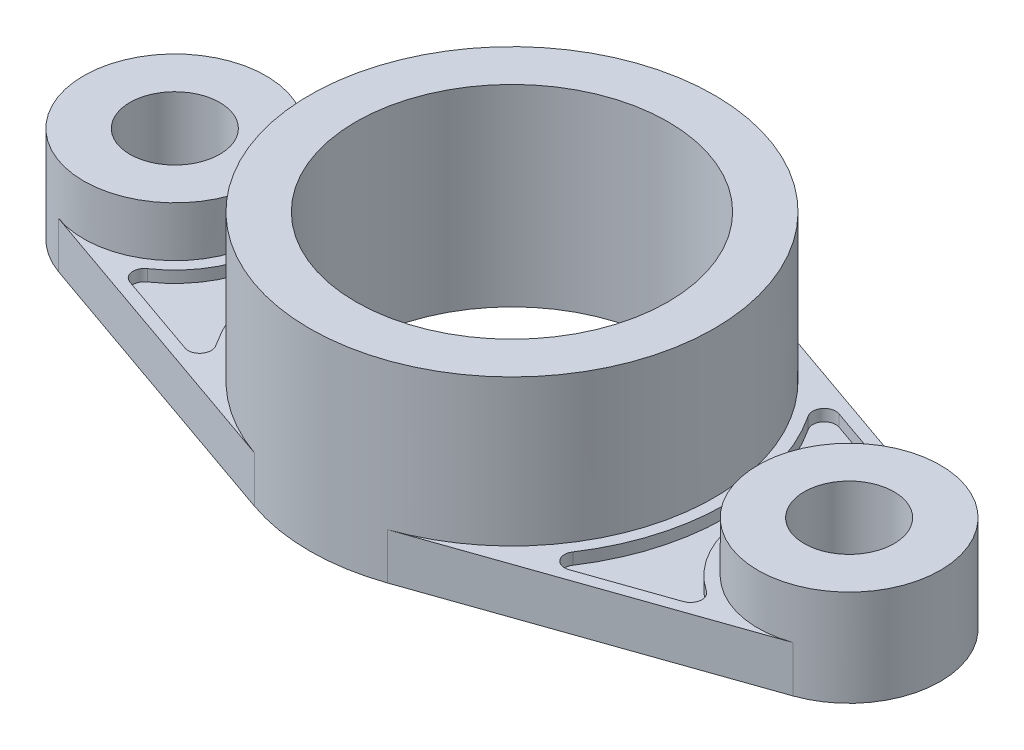
ISO-10303-21;
HEADER;
FILE_DESCRIPTION(('STEP AP214'),'2;1');
FILE_NAME('part.step','',(''),(''),'','','');
FILE_SCHEMA(('AUTOMOTIVE_DESIGN { 1 0 10303 214 1 1 1 1 }'));
ENDSEC;
DATA;
#1=APPLICATION_CONTEXT('core data for automotive mechanical design processes');
#2=APPLICATION_PROTOCOL_DEFINITION('international standard','automotive_design',2000,#1);
#3=PRODUCT_CONTEXT('',#1,'mechanical');
#4=PRODUCT('Part','Part','',(#3));
#5=PRODUCT_RELATED_PRODUCT_CATEGORY('part','',(#4));
#6=PRODUCT_DEFINITION_FORMATION('','',#4);
#7=PRODUCT_DEFINITION_CONTEXT('part definition',#1,'design');
#8=PRODUCT_DEFINITION('design','',#6,#7);
#9=PRODUCT_DEFINITION_SHAPE('','',#8);
#10=(LENGTH_UNIT() NAMED_UNIT(*) SI_UNIT(.MILLI.,.METRE.));
#11=(NAMED_UNIT(*) PLANE_ANGLE_UNIT() SI_UNIT($,.RADIAN.));
#12=(NAMED_UNIT(*) SI_UNIT($,.STERADIAN.) SOLID_ANGLE_UNIT());
#13=UNCERTAINTY_MEASURE_WITH_UNIT(LENGTH_MEASURE(1.E-05),#10,'distance_accuracy_value','');
#14=(GEOMETRIC_REPRESENTATION_CONTEXT(3) GLOBAL_UNCERTAINTY_ASSIGNED_CONTEXT((#13)) GLOBAL_UNIT_ASSIGNED_CONTEXT((#10,
#11,#12)) REPRESENTATION_CONTEXT('',''));
#15=CARTESIAN_POINT('',(0.,0.,0.));
#16=DIRECTION('',(0.,0.,1.));
#17=DIRECTION('',(1.,0.,0.));
#18=AXIS2_PLACEMENT_3D('',#15,#16,#17);
#19=CARTESIAN_POINT('',(0.,12.,0.));
#20=DIRECTION('',(0.,1.,0.));
#21=DIRECTION('',(0.,0.,1.));
#22=AXIS2_PLACEMENT_3D('',#19,#20,#21);
#23=PLANE('',#22);
#24=CARTESIAN_POINT('',(48.8374101689384,12.,32.2049276973396));
#25=DIRECTION('',(0.,1.,0.));
#26=DIRECTION('',(0.,0.,1.));
#27=AXIS2_PLACEMENT_3D('',#24,#25,#26);
#28=CIRCLE('',#27,3.00000000000001);
#29=CARTESIAN_POINT('',(46.3329275961723,12.,30.5533929436298));
#30=VERTEX_POINT('',#29);
#31=CARTESIAN_POINT('',(49.826038740367,12.,35.0373495493516));
#32=VERTEX_POINT('',#31);
#33=EDGE_CURVE('E59',#30,#32,#28,.T.);
#34=ORIENTED_EDGE('',*,*,#33,.F.);
#35=CARTESIAN_POINT('',(0.,12.,0.));
#36=DIRECTION('',(0.,-1.,0.));
#37=DIRECTION('',(0.,0.,1.));
#38=AXIS2_PLACEMENT_3D('',#35,#36,#37);
#39=CIRCLE('',#38,55.5);
#40=CARTESIAN_POINT('',(46.3329275961723,12.,-30.5533929436299));
#41=VERTEX_POINT('',#40);
#42=EDGE_CURVE('E223',#41,#30,#39,.T.);
#43=ORIENTED_EDGE('',*,*,#42,.F.);
#44=CARTESIAN_POINT('',(48.8374101689384,12.,-32.2049276973396));
#45=DIRECTION('',(0.,1.,0.));
#46=DIRECTION('',(0.,0.,1.));
#47=AXIS2_PLACEMENT_3D('',#44,#45,#46);
#48=CIRCLE('',#47,3.);
#49=CARTESIAN_POINT('',(49.826038740367,12.,-35.0373495493516));
#50=VERTEX_POINT('',#49);
#51=EDGE_CURVE('E229',#50,#41,#48,.T.);
#52=ORIENTED_EDGE('',*,*,#51,.F.);
#53=DIRECTION('',(-0.944140617337334,0.,-0.329542857142857));
#54=VECTOR('',#53,1.);
#55=CARTESIAN_POINT('',(71.8093276206941,12.,-27.3643020244494));
#56=LINE('',#55,#54);
#57=CARTESIAN_POINT('',(71.8093276206941,12.,-27.3643020244494));
#58=VERTEX_POINT('',#57);
#59=EDGE_CURVE('E258',#58,#50,#56,.T.);
#60=ORIENTED_EDGE('',*,*,#59,.F.);
#61=CARTESIAN_POINT('',(70.8206990492656,12.,-24.5318801724374));
#62=DIRECTION('',(0.,1.,0.));
#63=DIRECTION('',(0.,0.,1.));
#64=AXIS2_PLACEMENT_3D('',#61,#62,#63);
#65=CIRCLE('',#64,3.);
#66=CARTESIAN_POINT('',(72.507464694039,12.,-22.0509888689717));
#67=VERTEX_POINT('',#66);
#68=EDGE_CURVE('E251',#67,#58,#65,.T.);
#69=ORIENTED_EDGE('',*,*,#68,.F.);
#70=CARTESIAN_POINT('',(87.5,12.,0.));
#71=DIRECTION('',(0.,-1.,0.));
#72=DIRECTION('',(0.,0.,1.));
#73=AXIS2_PLACEMENT_3D('',#70,#71,#72);
#74=CIRCLE('',#73,26.665);
#75=CARTESIAN_POINT('',(72.5074646940389,12.,22.0509888689716));
#76=VERTEX_POINT('',#75);
#77=EDGE_CURVE('E249',#76,#67,#74,.T.);
#78=ORIENTED_EDGE('',*,*,#77,.F.);
#79=CARTESIAN_POINT('',(70.8206990492655,12.,24.5318801724374));
#80=DIRECTION('',(0.,1.,0.));
#81=DIRECTION('',(0.,0.,-1.));
#82=AXIS2_PLACEMENT_3D('',#79,#80,#81);
#83=CIRCLE('',#82,3.00000000000001);
#84=CARTESIAN_POINT('',(71.8093276206941,12.,27.3643020244494));
#85=VERTEX_POINT('',#84);
#86=EDGE_CURVE('E250',#85,#76,#83,.T.);
#87=ORIENTED_EDGE('',*,*,#86,.F.);
#88=DIRECTION('',(0.944140617337334,0.,-0.329542857142857));
#89=VECTOR('',#88,1.);
#90=CARTESIAN_POINT('',(49.826038740367,12.,35.0373495493516));
#91=LINE('',#90,#89);
#92=EDGE_CURVE('E245',#32,#85,#91,.T.);
#93=ORIENTED_EDGE('',*,*,#92,.F.);
#94=EDGE_LOOP('',(#34,#43,#52,#60,#69,#78,#87,#93));
#95=FACE_BOUND('',#94,.T.);
#96=CARTESIAN_POINT('',(87.5,12.,0.));
#97=DIRECTION('',(0.,1.,0.));
#98=DIRECTION('',(0.,0.,1.));
#99=AXIS2_PLACEMENT_3D('',#96,#97,#98);
#100=CIRCLE('',#99,23.665);
#101=CARTESIAN_POINT('',(95.2986317142857,12.,-22.343087709288));
#102=VERTEX_POINT('',#101);
#103=CARTESIAN_POINT('',(95.2986317142857,12.,22.343087709288));
#104=VERTEX_POINT('',#103);
#105=EDGE_CURVE('E340',#102,#104,#100,.T.);
#106=ORIENTED_EDGE('',*,*,#105,.F.);
#107=DIRECTION('',(0.944140617337334,0.,0.329542857142857));
#108=VECTOR('',#107,1.);
#109=CARTESIAN_POINT('',(17.301,12.,-49.56738241021));
#110=LINE('',#109,#108);
#111=CARTESIAN_POINT('',(17.301,12.,-49.56738241021));
#112=VERTEX_POINT('',#111);
#113=EDGE_CURVE('E366',#112,#102,#110,.T.);
#114=ORIENTED_EDGE('',*,*,#113,.F.);
#115=CARTESIAN_POINT('',(0.,12.,0.));
#116=DIRECTION('',(0.,1.,0.));
#117=DIRECTION('',(0.,0.,1.));
#118=AXIS2_PLACEMENT_3D('',#115,#116,#117);
#119=CIRCLE('',#118,52.5);
#120=CARTESIAN_POINT('',(17.301,12.,49.56738241021));
#121=VERTEX_POINT('',#120);
#122=EDGE_CURVE('E353',#121,#112,#119,.T.);
#123=ORIENTED_EDGE('',*,*,#122,.F.);
#124=DIRECTION('',(0.944140617337334,0.,-0.329542857142857));
#125=VECTOR('',#124,1.);
#126=CARTESIAN_POINT('',(17.301,12.,49.56738241021));
#127=LINE('',#126,#125);
#128=EDGE_CURVE('E365',#121,#104,#127,.T.);
#129=ORIENTED_EDGE('',*,*,#128,.T.);
#130=EDGE_LOOP('',(#106,#114,#123,#129));
#131=FACE_BOUND('',#130,.T.);
#132=ADVANCED_FACE('F41',(#95,#131),#23,.T.);
#133=CARTESIAN_POINT('',(-17.301,12.,49.56738241021));
#134=DIRECTION('',(-0.329542857142857,0.,0.944140617337334));
#135=DIRECTION('',(0.944140617337334,0.,0.329542857142857));
#136=AXIS2_PLACEMENT_3D('',#133,#134,#135);
#137=PLANE('',#136);
#138=DIRECTION('',(-0.944140617337334,0.,-0.329542857142857));
#139=VECTOR('',#138,1.);
#140=CARTESIAN_POINT('',(-17.301,0.,49.56738241021));
#141=LINE('',#140,#139);
#142=CARTESIAN_POINT('',(-17.301,0.,49.56738241021));
#143=VERTEX_POINT('',#142);
#144=CARTESIAN_POINT('',(-95.2986317142857,0.,22.343087709288));
#145=VERTEX_POINT('',#144);
#146=EDGE_CURVE('E380',#143,#145,#141,.T.);
#147=ORIENTED_EDGE('',*,*,#146,.F.);
#148=DIRECTION('',(0.,-1.,0.));
#149=VECTOR('',#148,1.);
#150=CARTESIAN_POINT('',(-17.301,12.,49.56738241021));
#151=LINE('',#150,#149);
#152=CARTESIAN_POINT('',(-17.301,12.,49.56738241021));
#153=VERTEX_POINT('',#152);
#154=EDGE_CURVE('E44',#153,#143,#151,.T.);
#155=ORIENTED_EDGE('',*,*,#154,.F.);
#156=DIRECTION('',(-0.944140617337334,0.,-0.329542857142857));
#157=VECTOR('',#156,1.);
#158=CARTESIAN_POINT('',(-17.301,12.,49.56738241021));
#159=LINE('',#158,#157);
#160=CARTESIAN_POINT('',(-95.2986317142857,12.,22.343087709288));
#161=VERTEX_POINT('',#160);
#162=EDGE_CURVE('E363',#153,#161,#159,.T.);
#163=ORIENTED_EDGE('',*,*,#162,.T.);
#164=DIRECTION('',(0.,-1.,0.));
#165=VECTOR('',#164,1.);
#166=CARTESIAN_POINT('',(-95.2986317142857,12.,22.343087709288));
#167=LINE('',#166,#165);
#168=EDGE_CURVE('E372',#161,#145,#167,.T.);
#169=ORIENTED_EDGE('',*,*,#168,.T.);
#170=EDGE_LOOP('',(#147,#155,#163,#169));
#171=FACE_BOUND('',#170,.T.);
#172=ADVANCED_FACE('F439',(#171),#137,.T.);
#173=CARTESIAN_POINT('',(17.301,12.,49.56738241021));
#174=DIRECTION('',(-0.329542857142857,0.,-0.944140617337334));
#175=DIRECTION('',(-0.944140617337334,0.,0.329542857142857));
#176=AXIS2_PLACEMENT_3D('',#173,#174,#175);
#177=PLANE('',#176);
#178=DIRECTION('',(0.944140617337334,0.,-0.329542857142857));
#179=VECTOR('',#178,1.);
#180=CARTESIAN_POINT('',(17.301,0.,49.56738241021));
#181=LINE('',#180,#179);
#182=CARTESIAN_POINT('',(17.301,0.,49.56738241021));
#183=VERTEX_POINT('',#182);
#184=CARTESIAN_POINT('',(95.2986317142857,0.,22.343087709288));
#185=VERTEX_POINT('',#184);
#186=EDGE_CURVE('E382',#183,#185,#181,.T.);
#187=ORIENTED_EDGE('',*,*,#186,.T.);
#188=DIRECTION('',(0.,-1.,0.));
#189=VECTOR('',#188,1.);
#190=CARTESIAN_POINT('',(95.2986317142857,12.,22.343087709288));
#191=LINE('',#190,#189);
#192=EDGE_CURVE('E414',#104,#185,#191,.T.);
#193=ORIENTED_EDGE('',*,*,#192,.F.);
#194=ORIENTED_EDGE('',*,*,#128,.F.);
#195=DIRECTION('',(0.,-1.,0.));
#196=VECTOR('',#195,1.);
#197=CARTESIAN_POINT('',(17.301,12.,49.56738241021));
#198=LINE('',#197,#196);
#199=EDGE_CURVE('E417',#121,#183,#198,.T.);
#200=ORIENTED_EDGE('',*,*,#199,.T.);
#201=EDGE_LOOP('',(#187,#193,#194,#200));
#202=FACE_BOUND('',#201,.T.);
#203=ADVANCED_FACE('F443',(#202),#177,.F.);
#204=CARTESIAN_POINT('',(87.5,12.,0.));
#205=DIRECTION('',(0.,-1.,0.));
#206=DIRECTION('',(0.,0.,-1.));
#207=AXIS2_PLACEMENT_3D('',#204,#205,#206);
#208=CYLINDRICAL_SURFACE('',#207,23.665);
#209=CARTESIAN_POINT('',(87.5,0.,0.));
#210=DIRECTION('',(0.,1.,0.));
#211=DIRECTION('',(0.,0.,1.));
#212=AXIS2_PLACEMENT_3D('',#209,#210,#211);
#213=CIRCLE('',#212,23.665);
#214=CARTESIAN_POINT('',(95.2986317142857,0.,-22.343087709288));
#215=VERTEX_POINT('',#214);
#216=EDGE_CURVE('E390',#185,#215,#213,.T.);
#217=ORIENTED_EDGE('',*,*,#216,.T.);
#218=DIRECTION('',(0.,-1.,0.));
#219=VECTOR('',#218,1.);
#220=CARTESIAN_POINT('',(95.2986317142857,12.,-22.343087709288));
#221=LINE('',#220,#219);
#222=EDGE_CURVE('E412',#102,#215,#221,.T.);
#223=ORIENTED_EDGE('',*,*,#222,.F.);
#224=ORIENTED_EDGE('',*,*,#105,.T.);
#225=ORIENTED_EDGE('',*,*,#192,.T.);
#226=EDGE_LOOP('',(#217,#223,#224,#225));
#227=FACE_BOUND('',#226,.T.);
#228=CARTESIAN_POINT('',(87.5,25.,0.));
#229=DIRECTION('',(0.,1.,0.));
#230=DIRECTION('',(0.,0.,1.));
#231=AXIS2_PLACEMENT_3D('',#228,#229,#230);
#232=CIRCLE('',#231,23.665);
#233=CARTESIAN_POINT('',(87.5,25.,23.665));
#234=VERTEX_POINT('',#233);
#235=EDGE_CURVE('E345',#234,#234,#232,.T.);
#236=ORIENTED_EDGE('',*,*,#235,.F.);
#237=EDGE_LOOP('',(#236));
#238=FACE_BOUND('',#237,.T.);
#239=ADVANCED_FACE('F453',(#227,#238),#208,.T.);
#240=CARTESIAN_POINT('',(17.301,12.,-49.56738241021));
#241=DIRECTION('',(0.329542857142857,0.,-0.944140617337334));
#242=DIRECTION('',(-0.944140617337334,0.,-0.329542857142857));
#243=AXIS2_PLACEMENT_3D('',#240,#241,#242);
#244=PLANE('',#243);
#245=DIRECTION('',(0.944140617337334,0.,0.329542857142857));
#246=VECTOR('',#245,1.);
#247=CARTESIAN_POINT('',(17.301,0.,-49.56738241021));
#248=LINE('',#247,#246);
#249=CARTESIAN_POINT('',(17.301,0.,-49.56738241021));
#250=VERTEX_POINT('',#249);
#251=EDGE_CURVE('E388',#250,#215,#248,.T.);
#252=ORIENTED_EDGE('',*,*,#251,.F.);
#253=DIRECTION('',(0.,-1.,0.));
#254=VECTOR('',#253,1.);
#255=CARTESIAN_POINT('',(17.301,12.,-49.56738241021));
#256=LINE('',#255,#254);
#257=EDGE_CURVE('E411',#112,#250,#256,.T.);
#258=ORIENTED_EDGE('',*,*,#257,.F.);
#259=ORIENTED_EDGE('',*,*,#113,.T.);
#260=ORIENTED_EDGE('',*,*,#222,.T.);
#261=EDGE_LOOP('',(#252,#258,#259,#260));
#262=FACE_BOUND('',#261,.T.);
#263=ADVANCED_FACE('F451',(#262),#244,.T.);
#264=CARTESIAN_POINT('',(0.,12.,0.));
#265=DIRECTION('',(0.,-1.,0.));
#266=DIRECTION('',(0.,0.,-1.));
#267=AXIS2_PLACEMENT_3D('',#264,#265,#266);
#268=CYLINDRICAL_SURFACE('',#267,52.5);
#269=CARTESIAN_POINT('',(0.,0.,0.));
#270=DIRECTION('',(0.,1.,0.));
#271=DIRECTION('',(0.,0.,1.));
#272=AXIS2_PLACEMENT_3D('',#269,#270,#271);
#273=CIRCLE('',#272,52.5);
#274=CARTESIAN_POINT('',(-17.301,0.,-49.56738241021));
#275=VERTEX_POINT('',#274);
#276=EDGE_CURVE('E383',#250,#275,#273,.T.);
#277=ORIENTED_EDGE('',*,*,#276,.T.);
#278=DIRECTION('',(0.,-1.,0.));
#279=VECTOR('',#278,1.);
#280=CARTESIAN_POINT('',(-17.301,12.,-49.56738241021));
#281=LINE('',#280,#279);
#282=CARTESIAN_POINT('',(-17.301,12.,-49.56738241021));
#283=VERTEX_POINT('',#282);
#284=EDGE_CURVE('E409',#283,#275,#281,.T.);
#285=ORIENTED_EDGE('',*,*,#284,.F.);
#286=EDGE_CURVE('E49',#283,#153,#119,.T.);
#287=ORIENTED_EDGE('',*,*,#286,.T.);
#288=ORIENTED_EDGE('',*,*,#154,.T.);
#289=EDGE_CURVE('E379',#143,#183,#273,.T.);
#290=ORIENTED_EDGE('',*,*,#289,.T.);
#291=ORIENTED_EDGE('',*,*,#199,.F.);
#292=ORIENTED_EDGE('',*,*,#122,.T.);
#293=ORIENTED_EDGE('',*,*,#257,.T.);
#294=EDGE_LOOP('',(#277,#285,#287,#288,#290,#291,#292,#293));
#295=FACE_BOUND('',#294,.T.);
#296=CARTESIAN_POINT('',(0.,50.,0.));
#297=DIRECTION('',(0.,1.,0.));
#298=DIRECTION('',(0.,0.,1.));
#299=AXIS2_PLACEMENT_3D('',#296,#297,#298);
#300=CIRCLE('',#299,52.5);
#301=CARTESIAN_POINT('',(0.,50.,52.5));
#302=VERTEX_POINT('',#301);
#303=EDGE_CURVE('E355',#302,#302,#300,.T.);
#304=ORIENTED_EDGE('',*,*,#303,.F.);
#305=EDGE_LOOP('',(#304));
#306=FACE_BOUND('',#305,.T.);
#307=ADVANCED_FACE('F426',(#295,#306),#268,.T.);
#308=CARTESIAN_POINT('',(-17.301,12.,-49.56738241021));
#309=DIRECTION('',(0.329542857142857,0.,0.944140617337334));
#310=DIRECTION('',(0.944140617337334,0.,-0.329542857142857));
#311=AXIS2_PLACEMENT_3D('',#308,#309,#310);
#312=PLANE('',#311);
#313=DIRECTION('',(-0.944140617337334,0.,0.329542857142857));
#314=VECTOR('',#313,1.);
#315=CARTESIAN_POINT('',(-17.301,0.,-49.56738241021));
#316=LINE('',#315,#314);
#317=CARTESIAN_POINT('',(-95.2986317142857,0.,-22.343087709288));
#318=VERTEX_POINT('',#317);
#319=EDGE_CURVE('E394',#275,#318,#316,.T.);
#320=ORIENTED_EDGE('',*,*,#319,.T.);
#321=DIRECTION('',(0.,-1.,0.));
#322=VECTOR('',#321,1.);
#323=CARTESIAN_POINT('',(-95.2986317142857,12.,-22.343087709288));
#324=LINE('',#323,#322);
#325=CARTESIAN_POINT('',(-95.2986317142857,12.,-22.343087709288));
#326=VERTEX_POINT('',#325);
#327=EDGE_CURVE('E403',#326,#318,#324,.T.);
#328=ORIENTED_EDGE('',*,*,#327,.F.);
#329=DIRECTION('',(-0.944140617337334,0.,0.329542857142857));
#330=VECTOR('',#329,1.);
#331=CARTESIAN_POINT('',(-17.301,12.,-49.56738241021));
#332=LINE('',#331,#330);
#333=EDGE_CURVE('E371',#283,#326,#332,.T.);
#334=ORIENTED_EDGE('',*,*,#333,.F.);
#335=ORIENTED_EDGE('',*,*,#284,.T.);
#336=EDGE_LOOP('',(#320,#328,#334,#335));
#337=FACE_BOUND('',#336,.T.);
#338=ADVANCED_FACE('F433',(#337),#312,.F.);
#339=CARTESIAN_POINT('',(0.,12.,0.));
#340=DIRECTION('',(0.,-1.,0.));
#341=DIRECTION('',(0.,0.,-1.));
#342=AXIS2_PLACEMENT_3D('',#339,#340,#341);
#343=CYLINDRICAL_SURFACE('',#342,40.5);
#344=CARTESIAN_POINT('',(0.,0.,0.));
#345=DIRECTION('',(0.,1.,0.));
#346=DIRECTION('',(0.,0.,1.));
#347=AXIS2_PLACEMENT_3D('',#344,#345,#346);
#348=CIRCLE('',#347,40.5);
#349=CARTESIAN_POINT('',(0.,0.,40.5));
#350=VERTEX_POINT('',#349);
#351=EDGE_CURVE('E398',#350,#350,#348,.T.);
#352=ORIENTED_EDGE('',*,*,#351,.F.);
#353=EDGE_LOOP('',(#352));
#354=FACE_BOUND('',#353,.T.);
#355=CARTESIAN_POINT('',(0.,50.,0.));
#356=DIRECTION('',(0.,1.,0.));
#357=DIRECTION('',(0.,0.,1.));
#358=AXIS2_PLACEMENT_3D('',#355,#356,#357);
#359=CIRCLE('',#358,40.5);
#360=CARTESIAN_POINT('',(0.,50.,40.5));
#361=VERTEX_POINT('',#360);
#362=EDGE_CURVE('E344',#361,#361,#359,.T.);
#363=ORIENTED_EDGE('',*,*,#362,.T.);
#364=EDGE_LOOP('',(#363));
#365=FACE_BOUND('',#364,.T.);
#366=ADVANCED_FACE('F706',(#354,#365),#343,.F.);
#367=CARTESIAN_POINT('',(-87.5,12.,0.));
#368=DIRECTION('',(0.,-1.,0.));
#369=DIRECTION('',(0.,0.,-1.));
#370=AXIS2_PLACEMENT_3D('',#367,#368,#369);
#371=CYLINDRICAL_SURFACE('',#370,23.665);
#372=CARTESIAN_POINT('',(-87.5,0.,0.));
#373=DIRECTION('',(0.,1.,0.));
#374=DIRECTION('',(0.,0.,1.));
#375=AXIS2_PLACEMENT_3D('',#372,#373,#374);
#376=CIRCLE('',#375,23.665);
#377=EDGE_CURVE('E396',#318,#145,#376,.T.);
#378=ORIENTED_EDGE('',*,*,#377,.T.);
#379=ORIENTED_EDGE('',*,*,#168,.F.);
#380=CARTESIAN_POINT('',(-87.5,12.,0.));
#381=DIRECTION('',(0.,1.,0.));
#382=DIRECTION('',(0.,0.,1.));
#383=AXIS2_PLACEMENT_3D('',#380,#381,#382);
#384=CIRCLE('',#383,23.665);
#385=EDGE_CURVE('E11',#161,#326,#384,.T.);
#386=ORIENTED_EDGE('',*,*,#385,.T.);
#387=ORIENTED_EDGE('',*,*,#327,.T.);
#388=EDGE_LOOP('',(#378,#379,#386,#387));
#389=FACE_BOUND('',#388,.T.);
#390=CARTESIAN_POINT('',(-87.5,25.,0.));
#391=DIRECTION('',(0.,1.,0.));
#392=DIRECTION('',(0.,0.,1.));
#393=AXIS2_PLACEMENT_3D('',#390,#391,#392);
#394=CIRCLE('',#393,23.665);
#395=CARTESIAN_POINT('',(-87.5,25.,23.665));
#396=VERTEX_POINT('',#395);
#397=EDGE_CURVE('E263',#396,#396,#394,.T.);
#398=ORIENTED_EDGE('',*,*,#397,.F.);
#399=EDGE_LOOP('',(#398));
#400=FACE_BOUND('',#399,.T.);
#401=ADVANCED_FACE('F434',(#389,#400),#371,.T.);
#402=CARTESIAN_POINT('',(-87.5,12.,0.));
#403=DIRECTION('',(0.,-1.,0.));
#404=DIRECTION('',(0.,0.,-1.));
#405=AXIS2_PLACEMENT_3D('',#402,#403,#404);
#406=CYLINDRICAL_SURFACE('',#405,11.665);
#407=CARTESIAN_POINT('',(-87.5,0.,0.));
#408=DIRECTION('',(0.,1.,0.));
#409=DIRECTION('',(0.,0.,1.));
#410=AXIS2_PLACEMENT_3D('',#407,#408,#409);
#411=CIRCLE('',#410,11.665);
#412=CARTESIAN_POINT('',(-87.5,0.,11.665));
#413=VERTEX_POINT('',#412);
#414=EDGE_CURVE('E357',#413,#413,#411,.T.);
#415=ORIENTED_EDGE('',*,*,#414,.F.);
#416=EDGE_LOOP('',(#415));
#417=FACE_BOUND('',#416,.T.);
#418=CARTESIAN_POINT('',(-87.5,25.,0.));
#419=DIRECTION('',(0.,1.,0.));
#420=DIRECTION('',(0.,0.,1.));
#421=AXIS2_PLACEMENT_3D('',#418,#419,#420);
#422=CIRCLE('',#421,11.665);
#423=CARTESIAN_POINT('',(-87.5,25.,11.665));
#424=VERTEX_POINT('',#423);
#425=EDGE_CURVE('E341',#424,#424,#422,.T.);
#426=ORIENTED_EDGE('',*,*,#425,.T.);
#427=EDGE_LOOP('',(#426));
#428=FACE_BOUND('',#427,.T.);
#429=ADVANCED_FACE('F43',(#417,#428),#406,.F.);
#430=CARTESIAN_POINT('',(87.5,12.,0.));
#431=DIRECTION('',(0.,-1.,0.));
#432=DIRECTION('',(0.,0.,-1.));
#433=AXIS2_PLACEMENT_3D('',#430,#431,#432);
#434=CYLINDRICAL_SURFACE('',#433,11.665);
#435=CARTESIAN_POINT('',(87.5,0.,0.));
#436=DIRECTION('',(0.,1.,0.));
#437=DIRECTION('',(0.,0.,1.));
#438=AXIS2_PLACEMENT_3D('',#435,#436,#437);
#439=CIRCLE('',#438,11.665);
#440=CARTESIAN_POINT('',(87.5,0.,11.665));
#441=VERTEX_POINT('',#440);
#442=EDGE_CURVE('E364',#441,#441,#439,.F.);
#443=ORIENTED_EDGE('',*,*,#442,.T.);
#444=EDGE_LOOP('',(#443));
#445=FACE_BOUND('',#444,.T.);
#446=CARTESIAN_POINT('',(87.5,25.,0.));
#447=DIRECTION('',(0.,1.,0.));
#448=DIRECTION('',(0.,0.,1.));
#449=AXIS2_PLACEMENT_3D('',#446,#447,#448);
#450=CIRCLE('',#449,11.665);
#451=CARTESIAN_POINT('',(87.5,25.,11.665));
#452=VERTEX_POINT('',#451);
#453=EDGE_CURVE('E337',#452,#452,#450,.T.);
#454=ORIENTED_EDGE('',*,*,#453,.T.);
#455=EDGE_LOOP('',(#454));
#456=FACE_BOUND('',#455,.T.);
#457=ADVANCED_FACE('F467',(#445,#456),#434,.F.);
#458=CARTESIAN_POINT('',(-70.8206990492656,12.,24.5318801724374));
#459=DIRECTION('',(0.,1.,0.));
#460=DIRECTION('',(0.,0.,1.));
#461=AXIS2_PLACEMENT_3D('',#458,#459,#460);
#462=CIRCLE('',#461,3.00000000000001);
#463=CARTESIAN_POINT('',(-72.507464694039,12.,22.0509888689717));
#464=VERTEX_POINT('',#463);
#465=CARTESIAN_POINT('',(-71.8093276206941,12.,27.3643020244494));
#466=VERTEX_POINT('',#465);
#467=EDGE_CURVE('E66',#464,#466,#462,.T.);
#468=ORIENTED_EDGE('',*,*,#467,.F.);
#469=CARTESIAN_POINT('',(-87.5,12.,0.));
#470=DIRECTION('',(0.,-1.,0.));
#471=DIRECTION('',(0.,0.,1.));
#472=AXIS2_PLACEMENT_3D('',#469,#470,#471);
#473=CIRCLE('',#472,26.665);
#474=CARTESIAN_POINT('',(-72.507464694039,12.,-22.0509888689717));
#475=VERTEX_POINT('',#474);
#476=EDGE_CURVE('E295',#475,#464,#473,.T.);
#477=ORIENTED_EDGE('',*,*,#476,.F.);
#478=CARTESIAN_POINT('',(-70.8206990492656,12.,-24.5318801724374));
#479=DIRECTION('',(0.,1.,0.));
#480=DIRECTION('',(0.,0.,-1.));
#481=AXIS2_PLACEMENT_3D('',#478,#479,#480);
#482=CIRCLE('',#481,3.);
#483=CARTESIAN_POINT('',(-71.8093276206941,12.,-27.3643020244494));
#484=VERTEX_POINT('',#483);
#485=EDGE_CURVE('E293',#484,#475,#482,.T.);
#486=ORIENTED_EDGE('',*,*,#485,.F.);
#487=DIRECTION('',(-0.944140617337334,0.,0.329542857142857));
#488=VECTOR('',#487,1.);
#489=CARTESIAN_POINT('',(-49.826038740367,12.,-35.0373495493516));
#490=LINE('',#489,#488);
#491=CARTESIAN_POINT('',(-49.826038740367,12.,-35.0373495493516));
#492=VERTEX_POINT('',#491);
#493=EDGE_CURVE('E298',#492,#484,#490,.T.);
#494=ORIENTED_EDGE('',*,*,#493,.F.);
#495=CARTESIAN_POINT('',(-48.8374101689384,12.,-32.2049276973396));
#496=DIRECTION('',(0.,1.,0.));
#497=DIRECTION('',(0.,0.,1.));
#498=AXIS2_PLACEMENT_3D('',#495,#496,#497);
#499=CIRCLE('',#498,3.00000000000001);
#500=CARTESIAN_POINT('',(-46.3329275961724,12.,-30.5533929436298));
#501=VERTEX_POINT('',#500);
#502=EDGE_CURVE('E305',#501,#492,#499,.T.);
#503=ORIENTED_EDGE('',*,*,#502,.F.);
#504=CARTESIAN_POINT('',(0.,12.,0.));
#505=DIRECTION('',(0.,-1.,0.));
#506=DIRECTION('',(0.,0.,1.));
#507=AXIS2_PLACEMENT_3D('',#504,#505,#506);
#508=CIRCLE('',#507,55.5);
#509=CARTESIAN_POINT('',(-46.3329275961724,12.,30.5533929436298));
#510=VERTEX_POINT('',#509);
#511=EDGE_CURVE('E304',#510,#501,#508,.T.);
#512=ORIENTED_EDGE('',*,*,#511,.F.);
#513=CARTESIAN_POINT('',(-48.8374101689385,12.,32.2049276973396));
#514=DIRECTION('',(0.,1.,0.));
#515=DIRECTION('',(0.,0.,1.));
#516=AXIS2_PLACEMENT_3D('',#513,#514,#515);
#517=CIRCLE('',#516,3.);
#518=CARTESIAN_POINT('',(-49.826038740367,12.,35.0373495493516));
#519=VERTEX_POINT('',#518);
#520=EDGE_CURVE('E306',#519,#510,#517,.T.);
#521=ORIENTED_EDGE('',*,*,#520,.F.);
#522=DIRECTION('',(0.944140617337334,0.,0.329542857142857));
#523=VECTOR('',#522,1.);
#524=CARTESIAN_POINT('',(-71.8093276206941,12.,27.3643020244494));
#525=LINE('',#524,#523);
#526=EDGE_CURVE('E313',#466,#519,#525,.T.);
#527=ORIENTED_EDGE('',*,*,#526,.F.);
#528=EDGE_LOOP('',(#468,#477,#486,#494,#503,#512,#521,#527));
#529=FACE_BOUND('',#528,.T.);
#530=ORIENTED_EDGE('',*,*,#385,.F.);
#531=ORIENTED_EDGE('',*,*,#162,.F.);
#532=ORIENTED_EDGE('',*,*,#286,.F.);
#533=ORIENTED_EDGE('',*,*,#333,.T.);
#534=EDGE_LOOP('',(#530,#531,#532,#533));
#535=FACE_BOUND('',#534,.T.);
#536=ADVANCED_FACE('F431',(#529,#535),#23,.T.);
#537=CARTESIAN_POINT('',(0.,0.,0.));
#538=DIRECTION('',(0.,1.,0.));
#539=DIRECTION('',(0.,0.,1.));
#540=AXIS2_PLACEMENT_3D('',#537,#538,#539);
#541=PLANE('',#540);
#542=ORIENTED_EDGE('',*,*,#414,.T.);
#543=EDGE_LOOP('',(#542));
#544=FACE_BOUND('',#543,.T.);
#545=ORIENTED_EDGE('',*,*,#146,.T.);
#546=ORIENTED_EDGE('',*,*,#377,.F.);
#547=ORIENTED_EDGE('',*,*,#319,.F.);
#548=ORIENTED_EDGE('',*,*,#276,.F.);
#549=ORIENTED_EDGE('',*,*,#251,.T.);
#550=ORIENTED_EDGE('',*,*,#216,.F.);
#551=ORIENTED_EDGE('',*,*,#186,.F.);
#552=ORIENTED_EDGE('',*,*,#289,.F.);
#553=EDGE_LOOP('',(#545,#546,#547,#548,#549,#550,#551,#552));
#554=FACE_BOUND('',#553,.T.);
#555=ORIENTED_EDGE('',*,*,#351,.T.);
#556=EDGE_LOOP('',(#555));
#557=FACE_BOUND('',#556,.T.);
#558=ORIENTED_EDGE('',*,*,#442,.F.);
#559=EDGE_LOOP('',(#558));
#560=FACE_BOUND('',#559,.T.);
#561=ADVANCED_FACE('F445',(#544,#554,#557,#560),#541,.F.);
#562=CARTESIAN_POINT('',(0.,50.,0.));
#563=DIRECTION('',(0.,1.,0.));
#564=DIRECTION('',(0.,0.,1.));
#565=AXIS2_PLACEMENT_3D('',#562,#563,#564);
#566=PLANE('',#565);
#567=ORIENTED_EDGE('',*,*,#303,.T.);
#568=EDGE_LOOP('',(#567));
#569=FACE_BOUND('',#568,.T.);
#570=ORIENTED_EDGE('',*,*,#362,.F.);
#571=EDGE_LOOP('',(#570));
#572=FACE_BOUND('',#571,.T.);
#573=ADVANCED_FACE('F488',(#569,#572),#566,.T.);
#574=CARTESIAN_POINT('',(-87.5,25.,0.));
#575=DIRECTION('',(0.,1.,0.));
#576=DIRECTION('',(0.,0.,1.));
#577=AXIS2_PLACEMENT_3D('',#574,#575,#576);
#578=PLANE('',#577);
#579=ORIENTED_EDGE('',*,*,#397,.T.);
#580=EDGE_LOOP('',(#579));
#581=FACE_BOUND('',#580,.T.);
#582=ORIENTED_EDGE('',*,*,#425,.F.);
#583=EDGE_LOOP('',(#582));
#584=FACE_BOUND('',#583,.T.);
#585=ADVANCED_FACE('F463',(#581,#584),#578,.T.);
#586=CARTESIAN_POINT('',(87.5,25.,0.));
#587=DIRECTION('',(0.,1.,0.));
#588=DIRECTION('',(0.,0.,1.));
#589=AXIS2_PLACEMENT_3D('',#586,#587,#588);
#590=PLANE('',#589);
#591=ORIENTED_EDGE('',*,*,#235,.T.);
#592=EDGE_LOOP('',(#591));
#593=FACE_BOUND('',#592,.T.);
#594=ORIENTED_EDGE('',*,*,#453,.F.);
#595=EDGE_LOOP('',(#594));
#596=FACE_BOUND('',#595,.T.);
#597=ADVANCED_FACE('F458',(#593,#596),#590,.T.);
#598=CARTESIAN_POINT('',(-70.8206990492656,9.,24.5318801724374));
#599=DIRECTION('',(0.,1.,0.));
#600=DIRECTION('',(0.,0.,1.));
#601=AXIS2_PLACEMENT_3D('',#598,#599,#600);
#602=CYLINDRICAL_SURFACE('',#601,3.00000000000001);
#603=ORIENTED_EDGE('',*,*,#467,.T.);
#604=DIRECTION('',(0.,1.,0.));
#605=VECTOR('',#604,1.);
#606=CARTESIAN_POINT('',(-71.8093276206941,9.,27.3643020244494));
#607=LINE('',#606,#605);
#608=CARTESIAN_POINT('',(-71.8093276206941,9.,27.3643020244494));
#609=VERTEX_POINT('',#608);
#610=EDGE_CURVE('E274',#609,#466,#607,.T.);
#611=ORIENTED_EDGE('',*,*,#610,.F.);
#612=CARTESIAN_POINT('',(-70.8206990492656,9.,24.5318801724374));
#613=DIRECTION('',(0.,1.,0.));
#614=DIRECTION('',(0.,0.,1.));
#615=AXIS2_PLACEMENT_3D('',#612,#613,#614);
#616=CIRCLE('',#615,3.00000000000001);
#617=CARTESIAN_POINT('',(-72.507464694039,9.,22.0509888689717));
#618=VERTEX_POINT('',#617);
#619=EDGE_CURVE('E296',#618,#609,#616,.T.);
#620=ORIENTED_EDGE('',*,*,#619,.F.);
#621=DIRECTION('',(0.,1.,0.));
#622=VECTOR('',#621,1.);
#623=CARTESIAN_POINT('',(-72.507464694039,9.,22.0509888689717));
#624=LINE('',#623,#622);
#625=EDGE_CURVE('E289',#618,#464,#624,.T.);
#626=ORIENTED_EDGE('',*,*,#625,.T.);
#627=EDGE_LOOP('',(#603,#611,#620,#626));
#628=FACE_BOUND('',#627,.T.);
#629=ADVANCED_FACE('F464',(#628),#602,.F.);
#630=CARTESIAN_POINT('',(-87.5,9.,0.));
#631=DIRECTION('',(0.,1.,0.));
#632=DIRECTION('',(0.,0.,1.));
#633=AXIS2_PLACEMENT_3D('',#630,#631,#632);
#634=CYLINDRICAL_SURFACE('',#633,26.665);
#635=ORIENTED_EDGE('',*,*,#476,.T.);
#636=ORIENTED_EDGE('',*,*,#625,.F.);
#637=CARTESIAN_POINT('',(-87.5,9.,0.));
#638=DIRECTION('',(0.,-1.,0.));
#639=DIRECTION('',(0.,0.,1.));
#640=AXIS2_PLACEMENT_3D('',#637,#638,#639);
#641=CIRCLE('',#640,26.665);
#642=CARTESIAN_POINT('',(-72.507464694039,9.,-22.0509888689717));
#643=VERTEX_POINT('',#642);
#644=EDGE_CURVE('E280',#643,#618,#641,.T.);
#645=ORIENTED_EDGE('',*,*,#644,.F.);
#646=DIRECTION('',(0.,1.,0.));
#647=VECTOR('',#646,1.);
#648=CARTESIAN_POINT('',(-72.507464694039,9.,-22.0509888689717));
#649=LINE('',#648,#647);
#650=EDGE_CURVE('E287',#643,#475,#649,.T.);
#651=ORIENTED_EDGE('',*,*,#650,.T.);
#652=EDGE_LOOP('',(#635,#636,#645,#651));
#653=FACE_BOUND('',#652,.T.);
#654=ADVANCED_FACE('F512',(#653),#634,.T.);
#655=CARTESIAN_POINT('',(-70.8206990492656,9.,-24.5318801724374));
#656=DIRECTION('',(0.,1.,0.));
#657=DIRECTION('',(0.,0.,1.));
#658=AXIS2_PLACEMENT_3D('',#655,#656,#657);
#659=CYLINDRICAL_SURFACE('',#658,3.);
#660=ORIENTED_EDGE('',*,*,#485,.T.);
#661=ORIENTED_EDGE('',*,*,#650,.F.);
#662=CARTESIAN_POINT('',(-70.8206990492656,9.,-24.5318801724374));
#663=DIRECTION('',(0.,1.,0.));
#664=DIRECTION('',(0.,0.,-1.));
#665=AXIS2_PLACEMENT_3D('',#662,#663,#664);
#666=CIRCLE('',#665,3.);
#667=CARTESIAN_POINT('',(-71.8093276206941,9.,-27.3643020244494));
#668=VERTEX_POINT('',#667);
#669=EDGE_CURVE('E320',#668,#643,#666,.T.);
#670=ORIENTED_EDGE('',*,*,#669,.F.);
#671=DIRECTION('',(0.,1.,0.));
#672=VECTOR('',#671,1.);
#673=CARTESIAN_POINT('',(-71.8093276206941,9.,-27.3643020244494));
#674=LINE('',#673,#672);
#675=EDGE_CURVE('E286',#668,#484,#674,.T.);
#676=ORIENTED_EDGE('',*,*,#675,.T.);
#677=EDGE_LOOP('',(#660,#661,#670,#676));
#678=FACE_BOUND('',#677,.T.);
#679=ADVANCED_FACE('F514',(#678),#659,.F.);
#680=CARTESIAN_POINT('',(-49.826038740367,9.,-35.0373495493516));
#681=DIRECTION('',(-0.329542857142857,0.,-0.944140617337334));
#682=DIRECTION('',(-0.944140617337334,0.,0.329542857142857));
#683=AXIS2_PLACEMENT_3D('',#680,#681,#682);
#684=PLANE('',#683);
#685=ORIENTED_EDGE('',*,*,#493,.T.);
#686=ORIENTED_EDGE('',*,*,#675,.F.);
#687=DIRECTION('',(-0.944140617337334,0.,0.329542857142857));
#688=VECTOR('',#687,1.);
#689=CARTESIAN_POINT('',(-49.826038740367,9.,-35.0373495493516));
#690=LINE('',#689,#688);
#691=CARTESIAN_POINT('',(-49.826038740367,9.,-35.0373495493516));
#692=VERTEX_POINT('',#691);
#693=EDGE_CURVE('E319',#692,#668,#690,.T.);
#694=ORIENTED_EDGE('',*,*,#693,.F.);
#695=DIRECTION('',(0.,1.,0.));
#696=VECTOR('',#695,1.);
#697=CARTESIAN_POINT('',(-49.826038740367,9.,-35.0373495493516));
#698=LINE('',#697,#696);
#699=EDGE_CURVE('E283',#692,#492,#698,.T.);
#700=ORIENTED_EDGE('',*,*,#699,.T.);
#701=EDGE_LOOP('',(#685,#686,#694,#700));
#702=FACE_BOUND('',#701,.T.);
#703=ADVANCED_FACE('F519',(#702),#684,.F.);
#704=CARTESIAN_POINT('',(-48.8374101689384,9.,-32.2049276973396));
#705=DIRECTION('',(0.,1.,0.));
#706=DIRECTION('',(0.,0.,1.));
#707=AXIS2_PLACEMENT_3D('',#704,#705,#706);
#708=CYLINDRICAL_SURFACE('',#707,3.00000000000001);
#709=ORIENTED_EDGE('',*,*,#502,.T.);
#710=ORIENTED_EDGE('',*,*,#699,.F.);
#711=CARTESIAN_POINT('',(-48.8374101689384,9.,-32.2049276973396));
#712=DIRECTION('',(0.,1.,0.));
#713=DIRECTION('',(0.,0.,1.));
#714=AXIS2_PLACEMENT_3D('',#711,#712,#713);
#715=CIRCLE('',#714,3.00000000000001);
#716=CARTESIAN_POINT('',(-46.3329275961724,9.,-30.5533929436298));
#717=VERTEX_POINT('',#716);
#718=EDGE_CURVE('E323',#717,#692,#715,.T.);
#719=ORIENTED_EDGE('',*,*,#718,.F.);
#720=DIRECTION('',(0.,1.,0.));
#721=VECTOR('',#720,1.);
#722=CARTESIAN_POINT('',(-46.3329275961724,9.,-30.5533929436298));
#723=LINE('',#722,#721);
#724=EDGE_CURVE('E282',#717,#501,#723,.T.);
#725=ORIENTED_EDGE('',*,*,#724,.T.);
#726=EDGE_LOOP('',(#709,#710,#719,#725));
#727=FACE_BOUND('',#726,.T.);
#728=ADVANCED_FACE('F525',(#727),#708,.F.);
#729=CARTESIAN_POINT('',(0.,9.,0.));
#730=DIRECTION('',(0.,1.,0.));
#731=DIRECTION('',(0.,0.,1.));
#732=AXIS2_PLACEMENT_3D('',#729,#730,#731);
#733=CYLINDRICAL_SURFACE('',#732,55.5);
#734=ORIENTED_EDGE('',*,*,#511,.T.);
#735=ORIENTED_EDGE('',*,*,#724,.F.);
#736=CARTESIAN_POINT('',(0.,9.,0.));
#737=DIRECTION('',(0.,-1.,0.));
#738=DIRECTION('',(0.,0.,1.));
#739=AXIS2_PLACEMENT_3D('',#736,#737,#738);
#740=CIRCLE('',#739,55.5);
#741=CARTESIAN_POINT('',(-46.3329275961724,9.,30.5533929436298));
#742=VERTEX_POINT('',#741);
#743=EDGE_CURVE('E326',#742,#717,#740,.T.);
#744=ORIENTED_EDGE('',*,*,#743,.F.);
#745=DIRECTION('',(0.,1.,0.));
#746=VECTOR('',#745,1.);
#747=CARTESIAN_POINT('',(-46.3329275961724,9.,30.5533929436298));
#748=LINE('',#747,#746);
#749=EDGE_CURVE('E278',#742,#510,#748,.T.);
#750=ORIENTED_EDGE('',*,*,#749,.T.);
#751=EDGE_LOOP('',(#734,#735,#744,#750));
#752=FACE_BOUND('',#751,.T.);
#753=ADVANCED_FACE('F528',(#752),#733,.T.);
#754=CARTESIAN_POINT('',(-48.8374101689385,9.,32.2049276973396));
#755=DIRECTION('',(0.,1.,0.));
#756=DIRECTION('',(0.,0.,1.));
#757=AXIS2_PLACEMENT_3D('',#754,#755,#756);
#758=CYLINDRICAL_SURFACE('',#757,3.);
#759=ORIENTED_EDGE('',*,*,#520,.T.);
#760=ORIENTED_EDGE('',*,*,#749,.F.);
#761=CARTESIAN_POINT('',(-48.8374101689385,9.,32.2049276973396));
#762=DIRECTION('',(0.,1.,0.));
#763=DIRECTION('',(0.,0.,1.));
#764=AXIS2_PLACEMENT_3D('',#761,#762,#763);
#765=CIRCLE('',#764,3.);
#766=CARTESIAN_POINT('',(-49.826038740367,9.,35.0373495493516));
#767=VERTEX_POINT('',#766);
#768=EDGE_CURVE('E328',#767,#742,#765,.T.);
#769=ORIENTED_EDGE('',*,*,#768,.F.);
#770=DIRECTION('',(0.,1.,0.));
#771=VECTOR('',#770,1.);
#772=CARTESIAN_POINT('',(-49.826038740367,9.,35.0373495493516));
#773=LINE('',#772,#771);
#774=EDGE_CURVE('E279',#767,#519,#773,.T.);
#775=ORIENTED_EDGE('',*,*,#774,.T.);
#776=EDGE_LOOP('',(#759,#760,#769,#775));
#777=FACE_BOUND('',#776,.T.);
#778=ADVANCED_FACE('F529',(#777),#758,.F.);
#779=CARTESIAN_POINT('',(-71.8093276206941,9.,27.3643020244494));
#780=DIRECTION('',(-0.329542857142857,0.,0.944140617337334));
#781=DIRECTION('',(0.944140617337334,0.,0.329542857142857));
#782=AXIS2_PLACEMENT_3D('',#779,#780,#781);
#783=PLANE('',#782);
#784=ORIENTED_EDGE('',*,*,#526,.T.);
#785=ORIENTED_EDGE('',*,*,#774,.F.);
#786=DIRECTION('',(0.944140617337334,0.,0.329542857142857));
#787=VECTOR('',#786,1.);
#788=CARTESIAN_POINT('',(-71.8093276206941,9.,27.3643020244494));
#789=LINE('',#788,#787);
#790=EDGE_CURVE('E335',#609,#767,#789,.T.);
#791=ORIENTED_EDGE('',*,*,#790,.F.);
#792=ORIENTED_EDGE('',*,*,#610,.T.);
#793=EDGE_LOOP('',(#784,#785,#791,#792));
#794=FACE_BOUND('',#793,.T.);
#795=ADVANCED_FACE('F508',(#794),#783,.F.);
#796=CARTESIAN_POINT('',(-70.8206990492656,9.,24.5318801724374));
#797=DIRECTION('',(0.,1.,0.));
#798=DIRECTION('',(0.,0.,1.));
#799=AXIS2_PLACEMENT_3D('',#796,#797,#798);
#800=PLANE('',#799);
#801=ORIENTED_EDGE('',*,*,#619,.T.);
#802=ORIENTED_EDGE('',*,*,#790,.T.);
#803=ORIENTED_EDGE('',*,*,#768,.T.);
#804=ORIENTED_EDGE('',*,*,#743,.T.);
#805=ORIENTED_EDGE('',*,*,#718,.T.);
#806=ORIENTED_EDGE('',*,*,#693,.T.);
#807=ORIENTED_EDGE('',*,*,#669,.T.);
#808=ORIENTED_EDGE('',*,*,#644,.T.);
#809=EDGE_LOOP('',(#801,#802,#803,#804,#805,#806,#807,#808));
#810=FACE_BOUND('',#809,.T.);
#811=ADVANCED_FACE('F506',(#810),#800,.T.);
#812=CARTESIAN_POINT('',(48.8374101689384,9.,32.2049276973396));
#813=DIRECTION('',(0.,1.,0.));
#814=DIRECTION('',(0.,0.,1.));
#815=AXIS2_PLACEMENT_3D('',#812,#813,#814);
#816=CYLINDRICAL_SURFACE('',#815,3.00000000000001);
#817=ORIENTED_EDGE('',*,*,#33,.T.);
#818=DIRECTION('',(0.,1.,0.));
#819=VECTOR('',#818,1.);
#820=CARTESIAN_POINT('',(49.826038740367,9.,35.0373495493516));
#821=LINE('',#820,#819);
#822=CARTESIAN_POINT('',(49.826038740367,9.,35.0373495493516));
#823=VERTEX_POINT('',#822);
#824=EDGE_CURVE('E205',#823,#32,#821,.T.);
#825=ORIENTED_EDGE('',*,*,#824,.F.);
#826=CARTESIAN_POINT('',(48.8374101689384,9.,32.2049276973396));
#827=DIRECTION('',(0.,1.,0.));
#828=DIRECTION('',(0.,0.,1.));
#829=AXIS2_PLACEMENT_3D('',#826,#827,#828);
#830=CIRCLE('',#829,3.00000000000001);
#831=CARTESIAN_POINT('',(46.3329275961723,9.,30.5533929436298));
#832=VERTEX_POINT('',#831);
#833=EDGE_CURVE('E206',#832,#823,#830,.T.);
#834=ORIENTED_EDGE('',*,*,#833,.F.);
#835=DIRECTION('',(0.,1.,0.));
#836=VECTOR('',#835,1.);
#837=CARTESIAN_POINT('',(46.3329275961723,9.,30.5533929436298));
#838=LINE('',#837,#836);
#839=EDGE_CURVE('E261',#832,#30,#838,.T.);
#840=ORIENTED_EDGE('',*,*,#839,.T.);
#841=EDGE_LOOP('',(#817,#825,#834,#840));
#842=FACE_BOUND('',#841,.T.);
#843=ADVANCED_FACE('F204',(#842),#816,.F.);
#844=CARTESIAN_POINT('',(0.,9.,0.));
#845=DIRECTION('',(0.,1.,0.));
#846=DIRECTION('',(0.,0.,1.));
#847=AXIS2_PLACEMENT_3D('',#844,#845,#846);
#848=CYLINDRICAL_SURFACE('',#847,55.5);
#849=ORIENTED_EDGE('',*,*,#42,.T.);
#850=ORIENTED_EDGE('',*,*,#839,.F.);
#851=CARTESIAN_POINT('',(0.,9.,0.));
#852=DIRECTION('',(0.,-1.,0.));
#853=DIRECTION('',(0.,0.,1.));
#854=AXIS2_PLACEMENT_3D('',#851,#852,#853);
#855=CIRCLE('',#854,55.5);
#856=CARTESIAN_POINT('',(46.3329275961723,9.,-30.5533929436299));
#857=VERTEX_POINT('',#856);
#858=EDGE_CURVE('E215',#857,#832,#855,.T.);
#859=ORIENTED_EDGE('',*,*,#858,.F.);
#860=DIRECTION('',(0.,1.,0.));
#861=VECTOR('',#860,1.);
#862=CARTESIAN_POINT('',(46.3329275961723,9.,-30.5533929436299));
#863=LINE('',#862,#861);
#864=EDGE_CURVE('E262',#857,#41,#863,.T.);
#865=ORIENTED_EDGE('',*,*,#864,.T.);
#866=EDGE_LOOP('',(#849,#850,#859,#865));
#867=FACE_BOUND('',#866,.T.);
#868=ADVANCED_FACE('F545',(#867),#848,.T.);
#869=CARTESIAN_POINT('',(48.8374101689384,9.,-32.2049276973396));
#870=DIRECTION('',(0.,1.,0.));
#871=DIRECTION('',(0.,0.,1.));
#872=AXIS2_PLACEMENT_3D('',#869,#870,#871);
#873=CYLINDRICAL_SURFACE('',#872,3.);
#874=ORIENTED_EDGE('',*,*,#51,.T.);
#875=ORIENTED_EDGE('',*,*,#864,.F.);
#876=CARTESIAN_POINT('',(48.8374101689384,9.,-32.2049276973396));
#877=DIRECTION('',(0.,1.,0.));
#878=DIRECTION('',(0.,0.,1.));
#879=AXIS2_PLACEMENT_3D('',#876,#877,#878);
#880=CIRCLE('',#879,3.);
#881=CARTESIAN_POINT('',(49.826038740367,9.,-35.0373495493516));
#882=VERTEX_POINT('',#881);
#883=EDGE_CURVE('E241',#882,#857,#880,.T.);
#884=ORIENTED_EDGE('',*,*,#883,.F.);
#885=DIRECTION('',(0.,1.,0.));
#886=VECTOR('',#885,1.);
#887=CARTESIAN_POINT('',(49.826038740367,9.,-35.0373495493516));
#888=LINE('',#887,#886);
#889=EDGE_CURVE('E266',#882,#50,#888,.T.);
#890=ORIENTED_EDGE('',*,*,#889,.T.);
#891=EDGE_LOOP('',(#874,#875,#884,#890));
#892=FACE_BOUND('',#891,.T.);
#893=ADVANCED_FACE('F560',(#892),#873,.F.);
#894=CARTESIAN_POINT('',(71.8093276206941,9.,-27.3643020244494));
#895=DIRECTION('',(0.329542857142857,0.,-0.944140617337334));
#896=DIRECTION('',(-0.944140617337334,0.,-0.329542857142857));
#897=AXIS2_PLACEMENT_3D('',#894,#895,#896);
#898=PLANE('',#897);
#899=ORIENTED_EDGE('',*,*,#59,.T.);
#900=ORIENTED_EDGE('',*,*,#889,.F.);
#901=DIRECTION('',(-0.944140617337334,0.,-0.329542857142857));
#902=VECTOR('',#901,1.);
#903=CARTESIAN_POINT('',(71.8093276206941,9.,-27.3643020244494));
#904=LINE('',#903,#902);
#905=CARTESIAN_POINT('',(71.8093276206941,9.,-27.3643020244494));
#906=VERTEX_POINT('',#905);
#907=EDGE_CURVE('E236',#906,#882,#904,.T.);
#908=ORIENTED_EDGE('',*,*,#907,.F.);
#909=DIRECTION('',(0.,1.,0.));
#910=VECTOR('',#909,1.);
#911=CARTESIAN_POINT('',(71.8093276206941,9.,-27.3643020244494));
#912=LINE('',#911,#910);
#913=EDGE_CURVE('E268',#906,#58,#912,.T.);
#914=ORIENTED_EDGE('',*,*,#913,.T.);
#915=EDGE_LOOP('',(#899,#900,#908,#914));
#916=FACE_BOUND('',#915,.T.);
#917=ADVANCED_FACE('F556',(#916),#898,.F.);
#918=CARTESIAN_POINT('',(70.8206990492656,9.,-24.5318801724374));
#919=DIRECTION('',(0.,1.,0.));
#920=DIRECTION('',(0.,0.,1.));
#921=AXIS2_PLACEMENT_3D('',#918,#919,#920);
#922=CYLINDRICAL_SURFACE('',#921,3.);
#923=ORIENTED_EDGE('',*,*,#68,.T.);
#924=ORIENTED_EDGE('',*,*,#913,.F.);
#925=CARTESIAN_POINT('',(70.8206990492656,9.,-24.5318801724374));
#926=DIRECTION('',(0.,1.,0.));
#927=DIRECTION('',(0.,0.,1.));
#928=AXIS2_PLACEMENT_3D('',#925,#926,#927);
#929=CIRCLE('',#928,3.);
#930=CARTESIAN_POINT('',(72.507464694039,9.,-22.0509888689717));
#931=VERTEX_POINT('',#930);
#932=EDGE_CURVE('E234',#931,#906,#929,.T.);
#933=ORIENTED_EDGE('',*,*,#932,.F.);
#934=DIRECTION('',(0.,1.,0.));
#935=VECTOR('',#934,1.);
#936=CARTESIAN_POINT('',(72.507464694039,9.,-22.0509888689717));
#937=LINE('',#936,#935);
#938=EDGE_CURVE('E269',#931,#67,#937,.T.);
#939=ORIENTED_EDGE('',*,*,#938,.T.);
#940=EDGE_LOOP('',(#923,#924,#933,#939));
#941=FACE_BOUND('',#940,.T.);
#942=ADVANCED_FACE('F555',(#941),#922,.F.);
#943=CARTESIAN_POINT('',(87.5,9.,0.));
#944=DIRECTION('',(0.,1.,0.));
#945=DIRECTION('',(0.,0.,1.));
#946=AXIS2_PLACEMENT_3D('',#943,#944,#945);
#947=CYLINDRICAL_SURFACE('',#946,26.665);
#948=ORIENTED_EDGE('',*,*,#77,.T.);
#949=ORIENTED_EDGE('',*,*,#938,.F.);
#950=CARTESIAN_POINT('',(87.5,9.,0.));
#951=DIRECTION('',(0.,-1.,0.));
#952=DIRECTION('',(0.,0.,1.));
#953=AXIS2_PLACEMENT_3D('',#950,#951,#952);
#954=CIRCLE('',#953,26.665);
#955=CARTESIAN_POINT('',(72.5074646940389,9.,22.0509888689716));
#956=VERTEX_POINT('',#955);
#957=EDGE_CURVE('E235',#956,#931,#954,.T.);
#958=ORIENTED_EDGE('',*,*,#957,.F.);
#959=DIRECTION('',(0.,1.,0.));
#960=VECTOR('',#959,1.);
#961=CARTESIAN_POINT('',(72.5074646940389,9.,22.0509888689716));
#962=LINE('',#961,#960);
#963=EDGE_CURVE('E275',#956,#76,#962,.T.);
#964=ORIENTED_EDGE('',*,*,#963,.T.);
#965=EDGE_LOOP('',(#948,#949,#958,#964));
#966=FACE_BOUND('',#965,.T.);
#967=ADVANCED_FACE('F547',(#966),#947,.T.);
#968=CARTESIAN_POINT('',(70.8206990492655,9.,24.5318801724374));
#969=DIRECTION('',(0.,1.,0.));
#970=DIRECTION('',(0.,0.,1.));
#971=AXIS2_PLACEMENT_3D('',#968,#969,#970);
#972=CYLINDRICAL_SURFACE('',#971,3.00000000000001);
#973=ORIENTED_EDGE('',*,*,#86,.T.);
#974=ORIENTED_EDGE('',*,*,#963,.F.);
#975=CARTESIAN_POINT('',(70.8206990492655,9.,24.5318801724374));
#976=DIRECTION('',(0.,1.,0.));
#977=DIRECTION('',(0.,0.,-1.));
#978=AXIS2_PLACEMENT_3D('',#975,#976,#977);
#979=CIRCLE('',#978,3.00000000000001);
#980=CARTESIAN_POINT('',(71.8093276206941,9.,27.3643020244494));
#981=VERTEX_POINT('',#980);
#982=EDGE_CURVE('E219',#981,#956,#979,.T.);
#983=ORIENTED_EDGE('',*,*,#982,.F.);
#984=DIRECTION('',(0.,1.,0.));
#985=VECTOR('',#984,1.);
#986=CARTESIAN_POINT('',(71.8093276206941,9.,27.3643020244494));
#987=LINE('',#986,#985);
#988=EDGE_CURVE('E211',#981,#85,#987,.T.);
#989=ORIENTED_EDGE('',*,*,#988,.T.);
#990=EDGE_LOOP('',(#973,#974,#983,#989));
#991=FACE_BOUND('',#990,.T.);
#992=ADVANCED_FACE('F544',(#991),#972,.F.);
#993=CARTESIAN_POINT('',(49.826038740367,9.,35.0373495493516));
#994=DIRECTION('',(0.329542857142857,0.,0.944140617337334));
#995=DIRECTION('',(0.944140617337334,0.,-0.329542857142857));
#996=AXIS2_PLACEMENT_3D('',#993,#994,#995);
#997=PLANE('',#996);
#998=ORIENTED_EDGE('',*,*,#92,.T.);
#999=ORIENTED_EDGE('',*,*,#988,.F.);
#1000=DIRECTION('',(0.944140617337334,0.,-0.329542857142857));
#1001=VECTOR('',#1000,1.);
#1002=CARTESIAN_POINT('',(49.826038740367,9.,35.0373495493516));
#1003=LINE('',#1002,#1001);
#1004=EDGE_CURVE('E214',#823,#981,#1003,.T.);
#1005=ORIENTED_EDGE('',*,*,#1004,.F.);
#1006=ORIENTED_EDGE('',*,*,#824,.T.);
#1007=EDGE_LOOP('',(#998,#999,#1005,#1006));
#1008=FACE_BOUND('',#1007,.T.);
#1009=ADVANCED_FACE('F216',(#1008),#997,.F.);
#1010=CARTESIAN_POINT('',(48.8374101689384,9.,32.2049276973396));
#1011=DIRECTION('',(0.,1.,0.));
#1012=DIRECTION('',(0.,0.,1.));
#1013=AXIS2_PLACEMENT_3D('',#1010,#1011,#1012);
#1014=PLANE('',#1013);
#1015=ORIENTED_EDGE('',*,*,#833,.T.);
#1016=ORIENTED_EDGE('',*,*,#1004,.T.);
#1017=ORIENTED_EDGE('',*,*,#982,.T.);
#1018=ORIENTED_EDGE('',*,*,#957,.T.);
#1019=ORIENTED_EDGE('',*,*,#932,.T.);
#1020=ORIENTED_EDGE('',*,*,#907,.T.);
#1021=ORIENTED_EDGE('',*,*,#883,.T.);
#1022=ORIENTED_EDGE('',*,*,#858,.T.);
#1023=EDGE_LOOP('',(#1015,#1016,#1017,#1018,#1019,#1020,#1021,#1022));
#1024=FACE_BOUND('',#1023,.T.);
#1025=ADVANCED_FACE('F225',(#1024),#1014,.T.);
#1026=CLOSED_SHELL('',(#132,#172,#203,#239,#263,#307,#338,#366,#401,#429,#457,#536,#561,#573,
#585,#597,#629,#654,#679,#703,#728,#753,#778,#795,#811,#843,#868,#893,#917,#942,#967,#992,#1009,#1025));
#1027=MANIFOLD_SOLID_BREP('B2',#1026);
#1028=ADVANCED_BREP_SHAPE_REPRESENTATION('',(#18,#1027),#14);
#1029=SHAPE_DEFINITION_REPRESENTATION(#9,#1028);
ENDSEC;
END-ISO-10303-21;
